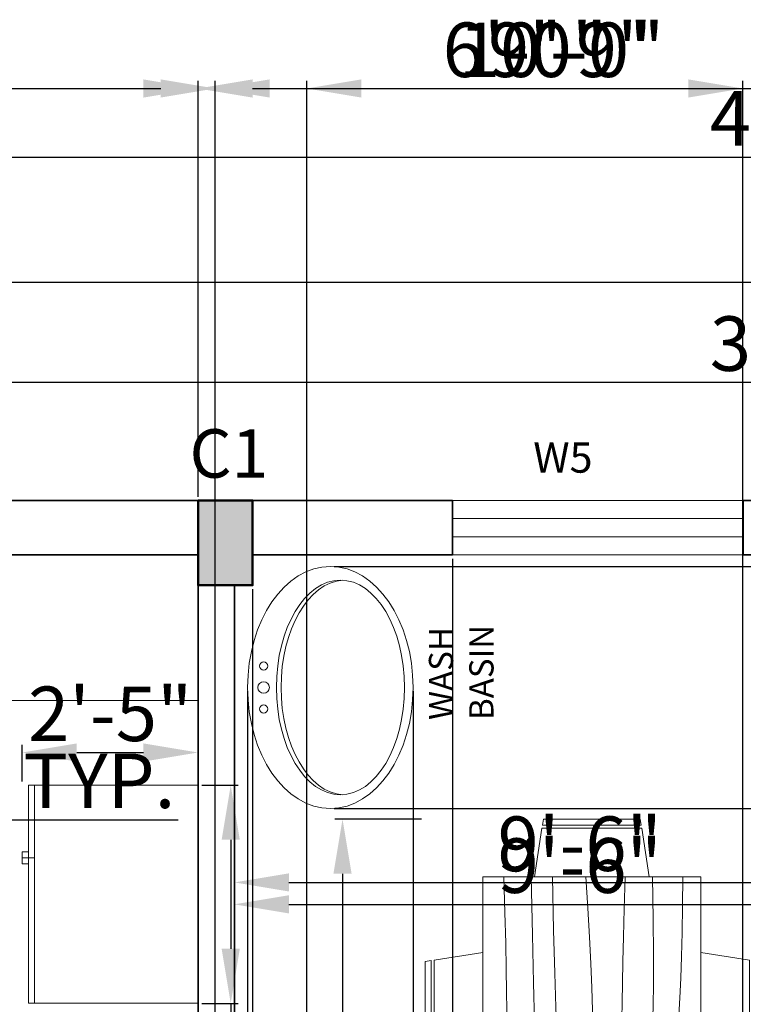
# Model space of a CAD drawing. Units: inches. Extents: x 2621 to 6190, y 513 to 1320.
# Tile 5 of 11: x 2878 to 2997, y 1003 to 1165. Entities that reach past the tile are written whole.
import ezdxf

# ---------------------------------------------------------------- set-up
doc = ezdxf.new("R2010")
doc.units = ezdxf.units.IN
for name, color, linetype, lineweight in [('A-ANNO-DIMS', 5, 'Continuous', 18), ('A-ANNO-TEXT', 7, 'Continuous', 18), ('A-EQPM', 30, 'Continuous', 13), ('A-FLOR-CASE', 30, 'Continuous', 18), ('A-FLOR-FIXT', 30, 'Continuous', 18), ('A-WALL', 7, 'Continuous', 35), ('C-PROP', 7, 'Continuous', 25), ('columns', 2, 'Continuous', 50), ('furniture', 30, 'Continuous', 18), ('S-COLS-IDEN', 2, 'Continuous', 25), ('S-COLS-PATT', 2, 'Continuous', 13), ('window', 172, 'Continuous', 18)]:
    doc.layers.add(name, color=color, linetype=linetype, lineweight=lineweight)
doc.styles.get("Standard").update_dxf_attribs({"font": 'arial.ttf'})
doc.dimstyles.new('ISO-25', dxfattribs={"dimtxt": 9, "dimasz": 9, "dimexe": 1.25, "dimexo": 0.625, "dimtad": 1, "dimlunit": 3, "dimtxsty": 'Standard', "dimcen": 2.5, "dimadec": 0, "dimazin": 0, "dimtfac": 1, "dimtmove": 0, "dimatfit": 3, "dimfxl": 1, "dimarcsym": 0})

# ---------------------------------------------------------------- blocks, each defined once
blk = doc.blocks.new('Dining Set - 36 x 72 in.')
for p, q in [((-22, 27.5), (-22.1562, 26.50042)), ((-5.8416, 26.5), (-22.1534, 26.5)), ((-22, 27.5), (-6, 27.5)), ((-5.8437, 26.49966), (-6, 27.5)), ((6, 27.5), (5.8438, 26.50042)), ((22.1584, 26.5), (5.8466, 26.5)), ((6, 27.5), (22, 27.5)), ((22.1563, 26.49966), (22, 27.5)), ((-22.2343, 26.00059), (-23.4847, 17.99762)), ((-22.2304, 26), (-5.7608, 26)), ((-4.5152, 17.99762), (-5.7655, 25.99926)), ((5.7657, 26.00059), (4.5153, 17.99762)), ((5.7696, 26), (22.2392, 26)), ((23.4848, 17.99762), (22.2345, 25.99926)), ((36, 18), (-36, 18)), ((-36, 18), (-36, -18)), ((36, -18), (36, 18)), ((-45.5, 8), (-44.5004, 8.15617)), ((-44.5, -8.15843), (-44.5, 8.15338)), ((-44.0006, 8.23428), (-35.9976, 9.48474)), ((-44, 8.23041), (-44, -8.23915)), ((44.0006, 8.23428), (35.9976, 9.48474)), ((44, 8.23041), (44, -8.23915)), ((44.5, -8.15843), (44.5, 8.15338)), ((45.5, 8), (44.5005, 8.15617)), ((-45.5, 8), (-45.5, -8)), ((45.5, 8), (45.5, -8)), ((-44.4997, -8.15631), (-45.5, -8)), ((44.4997, -8.15631), (45.5, -8)), ((-35.9976, -9.48476), (-43.9993, -8.2345)), ((35.9976, -9.48476), (43.9993, -8.2345)), ((-36, -18), (36, -18)), ((-22.2343, -26.0006), (-23.4847, -17.99762)), ((-4.5152, -17.99762), (-5.7655, -25.99928)), ((5.7657, -26.0006), (4.5153, -17.99762)), ((23.4848, -17.99762), (22.2345, -25.99928)), ((-22.2304, -26), (-5.7608, -26)), ((5.7696, -26), (22.2392, -26)), ((-22, -27.5), (-22.1562, -26.50044)), ((-5.8416, -26.5), (-22.1534, -26.5)), ((-22, -27.5), (-6, -27.5)), ((-5.8437, -26.49967), (-6, -27.5)), ((6, -27.5), (5.8438, -26.50044)), ((22.1584, -26.5), (5.8466, -26.5)), ((6, -27.5), (22, -27.5)), ((22.1563, -26.49967), (22, -27.5))]:
    blk.add_line(p, q)
for points in [[(-36, 15), (-31.1772, 14.97754), (-26.8079, 14.91406), (-22.8538, 14.81543), (-19.276, 14.6875), (-16.0362, 14.53613), (-13.0957, 14.36718), (-10.4159, 14.18652), (-7.9583, 14), (-5.6904, 13.81315), (-3.6035, 13.63021), (-1.6954, 13.45508), (0.0365, 13.29166), (1.5945, 13.14388), (2.9811, 13.01562), (4.1988, 12.9108), (5.25, 12.83333), (6.1393, 12.78613), (6.8802, 12.76823), (7.4883, 12.77767), (7.9792, 12.8125), (8.3685, 12.87077), (8.6719, 12.95052), (8.9049, 13.0498), (9.0833, 13.16666), (9.2205, 13.29899), (9.3216, 13.44401), (9.3895, 13.59879), (9.4271, 13.76041), (9.4373, 13.92594), (9.4232, 14.09245), (9.3875, 14.257), (9.3333, 14.41666), (9.2638, 14.56917), (9.1836, 14.71484), (9.0975, 14.85465), (9.0104, 14.98958), (8.9272, 15.1206), (8.8529, 15.2487), (8.7922, 15.37483), (8.75, 15.5), (8.7305, 15.62467), (8.7344, 15.74739), (8.7617, 15.86621), (8.8125, 15.97916), (8.8867, 16.08431), (8.9844, 16.17968), (9.1055, 16.26334), (9.25, 16.33333), (9.4189, 16.38802), (9.6172, 16.42708), (9.8506, 16.45052), (10.125, 16.45833), (10.4463, 16.45052), (10.8203, 16.42708), (11.2529, 16.38802), (11.75, 16.33333), (12.3184, 16.26318), (12.9694, 16.17838), (13.7151, 16.07991), (14.5677, 15.96875), (15.5395, 15.84586), (16.6426, 15.71224), (17.8893, 15.56884), (19.2917, 15.41666), (20.859, 15.25667), (22.5879, 15.08984), (24.4721, 14.91715), (26.5052, 14.73958), (28.6809, 14.5581), (30.9929, 14.3737), (33.4347, 14.18733), (36, 14)], [(-36, 10), (-28.9766, 10.14274), (-23.1725, 10.20442), (-18.4241, 10.19775), (-14.5677, 10.13541), (-11.4399, 10.03011), (-8.877, 9.89453), (-6.7154, 9.74137), (-4.7917, 9.58333), (-2.9698, 9.43082), (-1.2246, 9.28515), (0.4415, 9.14534), (2.026, 9.01041), (3.5266, 8.87939), (4.9408, 8.7513), (6.266, 8.62516), (7.5, 8.5), (8.6411, 8.37549), (9.6914, 8.2539), (10.6538, 8.13818), (11.5312, 8.03125), (12.3267, 7.93603), (13.043, 7.85547), (13.6831, 7.79248), (14.25, 7.75), (14.7471, 7.7303), (15.1797, 7.73307), (15.5537, 7.75732), (15.875, 7.80208), (16.1494, 7.86637), (16.3828, 7.94922), (16.5811, 8.04964), (16.75, 8.16666), (16.8944, 8.29915), (17.0143, 8.44531), (17.1089, 8.60319), (17.1771, 8.77083), (17.218, 8.94629), (17.2305, 9.1276), (17.2137, 9.31282), (17.1667, 9.5), (17.0895, 9.6875), (16.987, 9.875), (16.8649, 10.0625), (16.7292, 10.25), (16.5856, 10.4375), (16.4401, 10.625), (16.2985, 10.8125), (16.1667, 11), (16.05, 11.18733), (15.9518, 11.3737), (15.8752, 11.5581), (15.8229, 11.73958), (15.798, 11.91715), (15.8034, 12.08984), (15.842, 12.25667), (15.9167, 12.41666), (16.0295, 12.56836), (16.1784, 12.70833), (16.3605, 12.83268), (16.5729, 12.9375), (16.8127, 13.01888), (17.0768, 13.07291), (17.3625, 13.0957), (17.6667, 13.08333), (17.9894, 13.03312), (18.3418, 12.94726), (18.7382, 12.82918), (19.1927, 12.68229), (19.7195, 12.51001), (20.3327, 12.31575), (21.0465, 12.10294), (21.875, 11.875), (22.8357, 11.63354), (23.959, 11.37304), (25.2786, 11.08618), (26.8282, 10.76562), (28.6414, 10.40405), (30.752, 9.99414), (33.1936, 9.52856), (36, 9)], [(-36, 5.5), (-30.7157, 5.3348), (-26.069, 5.20963), (-21.9946, 5.11767), (-18.4271, 5.05208), (-15.3009, 5.00602), (-12.5508, 4.97265), (-10.1112, 4.94515), (-7.9167, 4.91666), (-5.909, 4.88167), (-4.0586, 4.83984), (-2.3429, 4.79215), (-0.7396, 4.73958), (0.7739, 4.6831), (2.22, 4.6237), (3.6213, 4.56233), (5, 4.5), (6.373, 4.43782), (7.7344, 4.3776), (9.0723, 4.32129), (10.375, 4.27083), (11.6309, 4.22819), (12.8281, 4.19531), (13.9551, 4.17415), (15, 4.16666), (15.954, 4.17448), (16.819, 4.19791), (17.6001, 4.23698), (18.3021, 4.29166), (18.9299, 4.36198), (19.4883, 4.44791), (19.9823, 4.54948), (20.4167, 4.66666), (20.7969, 4.79899), (21.1302, 4.94401), (21.4245, 5.09879), (21.6875, 5.26041), (21.9271, 5.42594), (22.1511, 5.59245), (22.3672, 5.757), (22.5834, 5.91666), (22.8065, 6.06868), (23.0404, 6.21093), (23.2879, 6.34147), (23.5521, 6.45833), (23.8358, 6.55957), (24.142, 6.64323), (24.4735, 6.70735), (24.8334, 6.75), (25.2235, 6.76969), (25.642, 6.76692), (26.0858, 6.74267), (26.5521, 6.69791), (27.0379, 6.63362), (27.5404, 6.55078), (28.0565, 6.45036), (28.5834, 6.33333), (29.1242, 6.19987), (29.7071, 6.04687), (30.3661, 5.87044), (31.1354, 5.66666), (32.0493, 5.43164), (33.142, 5.16146), (34.4475, 4.85221), (36, 4.5)], [(-36, -1), (-30.7915, -0.6591), (-26.0195, -0.38216), (-21.6519, -0.16284), (-17.6563, 0.00521), (-14.0005, 0.12833), (-10.6523, 0.21289), (-7.5796, 0.26522), (-4.75, 0.29166), (-2.134, 0.29793), (0.2878, 0.28711), (2.5317, 0.26163), (4.6146, 0.22396), (6.5529, 0.17651), (8.3633, 0.12174), (10.0623, 0.06209), (11.6667, 0), (13.1899, -0.06201), (14.6341, -0.1211), (15.9982, -0.17432), (17.2813, -0.21875), (18.4823, -0.25147), (19.6003, -0.26953), (20.6343, -0.27002), (21.5834, -0.25), (22.4481, -0.20768), (23.2357, -0.14584), (23.9549, -0.06836), (24.6146, 0.02083), (25.2235, 0.11784), (25.7904, 0.21875), (26.3241, 0.31966), (26.8334, 0.41666), (27.3265, 0.50618), (27.8099, 0.58593), (28.2894, 0.65397), (28.7709, 0.70833), (29.2601, 0.74707), (29.763, 0.76823), (30.2855, 0.76985), (30.8334, 0.75), (31.4088, 0.70784), (31.9994, 0.64713), (32.589, 0.57275), (33.1615, 0.48958), (33.7008, 0.4025), (34.1908, 0.3164), (34.6153, 0.23616), (34.9584, 0.16666), (35.2099, 0.11165), (35.3848, 0.07031), (35.504, 0.04069), (35.5886, 0.02083), (35.6594, 0.00879), (35.7377, 0.0026), (35.8442, 0.00032), (36, 0)], [(-36, -6.5), (-27.1843, -6.31267), (-20.084, -6.1263), (-14.469, -5.9419), (-10.1094, -5.76042), (-6.7752, -5.58285), (-4.2363, -5.41016), (-2.2629, -5.24333), (-0.625, -5.08334), (0.8708, -4.93099), (2.2715, -4.78646), (3.5872, -4.64974), (4.8281, -4.52084), (6.0046, -4.39974), (7.127, -4.28646), (8.2053, -4.18099), (9.25, -4.08334), (10.2705, -3.99382), (11.2734, -3.91407), (12.2647, -3.84603), (13.25, -3.79167), (14.2354, -3.75293), (15.2266, -3.73177), (16.2295, -3.73015), (17.25, -3.75), (18.2912, -3.79248), (19.3451, -3.85547), (20.4009, -3.93604), (21.4479, -4.03125), (22.4754, -4.13819), (23.4727, -4.25391), (24.4289, -4.37549), (25.3334, -4.5), (26.1785, -4.62492), (26.9694, -4.74935), (27.7145, -4.87281), (28.4219, -4.99479), (29.1, -5.11483), (29.7572, -5.23242), (30.4016, -5.34709), (31.0417, -5.45834), (31.6837, -5.56437), (32.3262, -5.65821), (32.9658, -5.73153), (33.599, -5.77604), (34.2224, -5.78345), (34.8327, -5.74545), (35.4264, -5.65373), (36, -5.5)], [(-36, -10), (-26.4022, -9.81299), (-18.4675, -9.62891), (-11.9839, -9.45069), (-6.7396, -9.28125), (-2.5226, -9.12354), (0.8789, -8.98047), (3.6769, -8.85498), (6.0833, -8.75), (8.2767, -8.66765), (10.3021, -8.60677), (12.1712, -8.56543), (13.8958, -8.54167), (15.4876, -8.53353), (16.9583, -8.53907), (18.3197, -8.55632), (19.5834, -8.58334), (20.7616, -8.61841), (21.8685, -8.66081), (22.9188, -8.71004), (23.9271, -8.76563), (24.9081, -8.82707), (25.8763, -8.89388), (26.8465, -8.96558), (27.8334, -9.04167), (28.8474, -9.12118), (29.8828, -9.20117), (30.93, -9.27824), (31.9792, -9.34896), (33.0205, -9.40991), (34.0443, -9.45768), (35.0407, -9.48885), (36, -9.5)], [(-36, -14.5), (-30.0881, -14.33513), (-25.0332, -14.21224), (-20.7312, -14.12647), (-17.0781, -14.07292), (-13.97, -14.04671), (-11.3027, -14.04297), (-8.9724, -14.05681), (-6.875, -14.08334), (-4.9224, -14.11833), (-3.0905, -14.16016), (-1.3709, -14.20785), (0.2448, -14.26042), (1.7647, -14.3169), (3.1973, -14.3763), (4.5507, -14.43767), (5.8333, -14.5), (7.0554, -14.5621), (8.235, -14.62175), (9.3922, -14.67652), (10.5469, -14.72396), (11.7192, -14.76164), (12.929, -14.78711), (14.1965, -14.79794), (15.5417, -14.79167), (16.9933, -14.76424), (18.6152, -14.70508), (20.4804, -14.60197), (22.6615, -14.44271), (25.2312, -14.21509), (28.2624, -13.9069), (31.8277, -13.50594), (36, -13)]]:
    blk.add_lwpolyline(points)
blk = doc.blocks.new('Refrigerator-2 door - 36 in top')
for p, q in [((0, -26.999999), (36, -26.999999)), ((12, -26.999999), (12, -28.999999)), ((11, -27.999999), (11, -28.999999)), ((11, -28.999999), (13, -28.999999)), ((13, -28.999999), (13, -27.999999))]:
    blk.add_line(p, q)
blk.add_lwpolyline([(0, -27.999999), (0, 0), (36, 0), (36, -27.999999)], close=True)
blk = doc.blocks.new('*D20')
at = {"layer": 'A-ANNO-DIMS', "color": 0, "lineweight": -2, "transparency": 16777216}
for p, q in [((2913.38, 1018.55), (2913.38, 1020.48)), ((2922.38, 1019.23), (3018.38, 1019.23)), ((3027.38, 1018.55), (3027.38, 1020.48))]:
    blk.add_line(p, q, dxfattribs=at)
at = {"layer": 'A-ANNO-DIMS', "color": 0, "transparency": 16777216}
for points in [[(2922.38, 1020.73), (2922.38, 1017.73), (2913.38, 1019.23)], [(3018.38, 1020.73), (3018.38, 1017.73), (3027.38, 1019.23)]]:
    blk.add_solid(points, dxfattribs=at)
at = {"layer": 'Defpoints', "color": 0, "transparency": 16777216}
for p in [(3027.38, 1019.23), (2913.38, 1017.92), (3027.38, 1017.92)]:
    blk.add_point(p, dxfattribs=at)
at = {"layer": 'A-ANNO-DIMS', "color": 0, "transparency": 16777216, "insert": (2970.38, 1024.45), "char_height": 9, "attachment_point": 5}
blk.add_mtext('9\'-6"', dxfattribs=at)
blk = doc.blocks.new('*D21')
at = {"layer": 'A-ANNO-DIMS', "color": 0, "lineweight": -2, "transparency": 16777216}
for p, q in [((2913.38, 1022.82), (2913.38, 1024.1)), ((3027.38, 1022.82), (3027.38, 1024.1)), ((2922.38, 1022.85), (3018.38, 1022.85))]:
    blk.add_line(p, q, dxfattribs=at)
at = {"layer": 'A-ANNO-DIMS', "color": 0, "transparency": 16777216}
for points in [[(2922.38, 1024.35), (2922.38, 1021.35), (2913.38, 1022.85)], [(3018.38, 1024.35), (3018.38, 1021.35), (3027.38, 1022.85)]]:
    blk.add_solid(points, dxfattribs=at)
at = {"layer": 'Defpoints', "color": 0, "transparency": 16777216}
for p in [(3027.38, 1022.85), (2913.38, 1022.19), (3027.38, 1022.19)]:
    blk.add_point(p, dxfattribs=at)
at = {"layer": 'A-ANNO-DIMS', "color": 0, "transparency": 16777216, "insert": (2970.38, 1028.07), "char_height": 9, "attachment_point": 5}
blk.add_mtext('9\'-6"', dxfattribs=at)
blk = doc.blocks.new('*D36')
at = {"layer": 'A-ANNO-DIMS', "color": 0, "lineweight": -2, "transparency": 16777216}
for p, q in [((2778.38, 1086.51), (2778.38, 1106.64)), ((2787.38, 1105.39), (3213.38, 1105.39)), ((3222.38, 1086.51), (3222.38, 1106.64))]:
    blk.add_line(p, q, dxfattribs=at)
at = {"layer": 'A-ANNO-DIMS', "color": 0, "transparency": 16777216}
for points in [[(2787.38, 1106.89), (2787.38, 1103.89), (2778.38, 1105.39)], [(3213.38, 1106.89), (3213.38, 1103.89), (3222.38, 1105.39)]]:
    blk.add_solid(points, dxfattribs=at)
at = {"layer": 'Defpoints', "color": 0, "transparency": 16777216}
for p in [(3222.38, 1105.39), (2778.38, 1085.89), (3222.38, 1085.89)]:
    blk.add_point(p, dxfattribs=at)
at = {"layer": 'A-ANNO-DIMS', "color": 0, "transparency": 16777216, "insert": (3000.38, 1110.61), "char_height": 9, "attachment_point": 5}
blk.add_mtext("37'", dxfattribs=at)
blk = doc.blocks.new('*D38')
at = {"layer": 'A-ANNO-DIMS', "color": 0, "lineweight": -2, "transparency": 16777216}
for p, q in [((2742.38, 1122.51), (2742.38, 1143.81)), ((2751.38, 1142.56), (3249.38, 1142.56)), ((3258.38, 1122.51), (3258.38, 1143.81))]:
    blk.add_line(p, q, dxfattribs=at)
at = {"layer": 'A-ANNO-DIMS', "color": 0, "transparency": 16777216}
for points in [[(2751.38, 1144.06), (2751.38, 1141.06), (2742.38, 1142.56)], [(3249.38, 1144.06), (3249.38, 1141.06), (3258.38, 1142.56)]]:
    blk.add_solid(points, dxfattribs=at)
at = {"layer": 'Defpoints', "color": 0, "transparency": 16777216}
for p in [(3258.38, 1142.56), (2742.38, 1121.89), (3258.38, 1121.89)]:
    blk.add_point(p, dxfattribs=at)
at = {"layer": 'A-ANNO-DIMS', "color": 0, "transparency": 16777216, "insert": (3000.38, 1147.79), "char_height": 9, "attachment_point": 5}
blk.add_mtext("43'", dxfattribs=at)
blk = doc.blocks.new('WIN-48IN')
for p, q in [((48, 9), (0, 9)), ((0, 9), (0, 0)), ((48, 0), (48, 9)), ((0, 6), (48, 6)), ((0, 3), (48, 3)), ((0, 0), (48, 0))]:
    blk.add_line(p, q)
blk = doc.blocks.new('COL-C1-9X14')
blk.add_lwpolyline([(0, 0), (0, 9), (14, 9), (14, 0)], close=True)
blk = doc.blocks.new('*D68')
at = {"layer": 'A-ANNO-DIMS', "color": 0, "lineweight": -2, "transparency": 16777216}
for p, q in [((2807.53, 1033.24), (2807.53, 1034.43)), ((2809.04, 1033.24), (2809.04, 1034.43)), ((2798.53, 1033.18), (2789.53, 1033.18)), ((2807.53, 1033.18), (2809.04, 1033.18)), ((2818.04, 1033.18), (2904.12, 1033.18))]:
    blk.add_line(p, q, dxfattribs=at)
at = {"layer": 'A-ANNO-DIMS', "color": 0, "transparency": 16777216}
for points in [[(2798.53, 1034.68), (2798.53, 1031.68), (2807.53, 1033.18)], [(2818.04, 1034.68), (2818.04, 1031.68), (2809.04, 1033.18)]]:
    blk.add_solid(points, dxfattribs=at)
at = {"layer": 'Defpoints', "color": 0, "transparency": 16777216}
for p in [(2807.53, 1032.61), (2809.04, 1033.18), (2809.04, 1032.61)]:
    blk.add_point(p, dxfattribs=at)
at = {"layer": 'A-ANNO-DIMS', "color": 0, "transparency": 16777216, "insert": (2865.58, 1038.46), "char_height": 9, "attachment_point": 5}
blk.add_mtext('0\'-1 1/2" TYP.', dxfattribs=at)
blk = doc.blocks.new('*D73')
at = {"layer": 'A-ANNO-DIMS', "color": 0, "lineweight": -2, "transparency": 16777216}
for p, q in [((2944.26, 1033.29), (2929.98, 1033.29)), ((2931.23, 1024.29), (2931.23, 951.29)), ((2944.26, 942.29), (2929.98, 942.29)), ((2931.23, 942.29), (2931.23, 833.12))]:
    blk.add_line(p, q, dxfattribs=at)
at = {"layer": 'A-ANNO-DIMS', "color": 0, "transparency": 16777216}
for points in [[(2929.73, 1024.29), (2932.73, 1024.29), (2931.23, 1033.29)], [(2929.73, 951.29), (2932.73, 951.29), (2931.23, 942.29)]]:
    blk.add_solid(points, dxfattribs=at)
at = {"layer": 'Defpoints', "color": 0, "transparency": 16777216}
for p in [(2944.88, 1033.29), (2931.23, 942.29), (2944.88, 942.29)]:
    blk.add_point(p, dxfattribs=at)
at = {"layer": 'A-ANNO-DIMS', "color": 0, "transparency": 16777216, "insert": (2925.95, 883.21), "char_height": 9, "attachment_point": 5, "rotation": 90}
blk.add_mtext('DINING SET 7\'-7"', dxfattribs=at)
blk = doc.blocks.new('*D75')
at = {"layer": 'A-ANNO-DIMS', "color": 0, "lineweight": -2, "transparency": 16777216}
for p, q in [((2908.01, 1038.89), (2914.03, 1038.89)), ((2912.78, 1029.89), (2912.78, 1011.89)), ((2908.01, 1002.89), (2914.03, 1002.89)), ((2912.78, 1002.89), (2912.78, 918.24))]:
    blk.add_line(p, q, dxfattribs=at)
at = {"layer": 'A-ANNO-DIMS', "color": 0, "transparency": 16777216}
for points in [[(2911.28, 1029.89), (2914.28, 1029.89), (2912.78, 1038.89)], [(2911.28, 1011.89), (2914.28, 1011.89), (2912.78, 1002.89)]]:
    blk.add_solid(points, dxfattribs=at)
at = {"layer": 'Defpoints', "color": 0, "transparency": 16777216}
for p in [(2907.38, 1038.89), (2907.38, 1002.89), (2912.78, 1002.89)]:
    blk.add_point(p, dxfattribs=at)
at = {"layer": 'A-ANNO-DIMS', "color": 0, "transparency": 16777216, "insert": (2907.5, 956.07), "char_height": 9, "attachment_point": 5, "rotation": 90}
blk.add_mtext('FRIDGE 3\'-0"', dxfattribs=at)
blk = doc.blocks.new('*D76')
at = {"layer": 'A-ANNO-DIMS', "color": 0, "lineweight": -2, "transparency": 16777216}
for p, q in [((2878.38, 1039.52), (2878.38, 1045.54)), ((2907.38, 1039.52), (2907.38, 1045.54)), ((2887.38, 1044.29), (2898.38, 1044.29))]:
    blk.add_line(p, q, dxfattribs=at)
at = {"layer": 'A-ANNO-DIMS', "color": 0, "transparency": 16777216}
for points in [[(2887.38, 1045.79), (2887.38, 1042.79), (2878.38, 1044.29)], [(2898.38, 1045.79), (2898.38, 1042.79), (2907.38, 1044.29)]]:
    blk.add_solid(points, dxfattribs=at)
at = {"layer": 'Defpoints', "color": 0, "transparency": 16777216}
for p in [(2907.38, 1044.29), (2878.38, 1038.89), (2907.38, 1038.89)]:
    blk.add_point(p, dxfattribs=at)
at = {"layer": 'A-ANNO-DIMS', "color": 0, "transparency": 16777216, "insert": (2892.88, 1049.51), "char_height": 9, "attachment_point": 5}
blk.add_mtext('2\'-5"', dxfattribs=at)
blk = doc.blocks.new('*D79')
at = {"layer": 'A-ANNO-DIMS', "color": 0, "lineweight": -2, "transparency": 16777216}
for p, q in [((2778.38, 1086.51), (2778.38, 1155.14)), ((2787.38, 1153.89), (2898.38, 1153.89)), ((2907.38, 1086.51), (2907.38, 1155.14))]:
    blk.add_line(p, q, dxfattribs=at)
at = {"layer": 'A-ANNO-DIMS', "color": 0, "transparency": 16777216}
for points in [[(2787.38, 1155.39), (2787.38, 1152.39), (2778.38, 1153.89)], [(2898.38, 1155.39), (2898.38, 1152.39), (2907.38, 1153.89)]]:
    blk.add_solid(points, dxfattribs=at)
at = {"layer": 'Defpoints', "color": 0, "transparency": 16777216}
for p in [(2907.38, 1153.89), (2778.38, 1085.89), (2907.38, 1085.89)]:
    blk.add_point(p, dxfattribs=at)
at = {"layer": 'A-ANNO-DIMS', "color": 0, "transparency": 16777216, "insert": (2842.88, 1159.11), "char_height": 9, "attachment_point": 5}
blk.add_mtext('10\'-9"', dxfattribs=at)
blk = doc.blocks.new('*D80')
at = {"layer": 'A-ANNO-DIMS', "color": 0, "lineweight": -2, "transparency": 16777216}
for p, q in [((2907.38, 1086.51), (2907.38, 1155.14)), ((2916.38, 1153.89), (3018.38, 1153.89)), ((3027.38, 1086.51), (3027.38, 1155.14))]:
    blk.add_line(p, q, dxfattribs=at)
at = {"layer": 'A-ANNO-DIMS', "color": 0, "transparency": 16777216}
for points in [[(2916.38, 1155.39), (2916.38, 1152.39), (2907.38, 1153.89)], [(3018.38, 1155.39), (3018.38, 1152.39), (3027.38, 1153.89)]]:
    blk.add_solid(points, dxfattribs=at)
at = {"layer": 'Defpoints', "color": 0, "transparency": 16777216}
for p in [(3027.38, 1153.89), (2907.38, 1085.89), (3027.38, 1085.89)]:
    blk.add_point(p, dxfattribs=at)
at = {"layer": 'A-ANNO-DIMS', "color": 0, "transparency": 16777216, "insert": (2967.38, 1159.11), "char_height": 9, "attachment_point": 5}
blk.add_mtext('10\'-0"', dxfattribs=at)
blk = doc.blocks.new('*D87')
at = {"layer": 'A-ANNO-DIMS', "color": 0, "lineweight": -2, "transparency": 16777216}
for p, q in [((2778.38, 897.51), (2778.38, 1155.14)), ((2787.38, 1153.89), (2901.22, 1153.89)), ((2910.22, 898.87), (2910.22, 1155.14))]:
    blk.add_line(p, q, dxfattribs=at)
at = {"layer": 'A-ANNO-DIMS', "color": 0, "transparency": 16777216}
for points in [[(2787.38, 1155.39), (2787.38, 1152.39), (2778.38, 1153.89)], [(2901.22, 1155.39), (2901.22, 1152.39), (2910.22, 1153.89)]]:
    blk.add_solid(points, dxfattribs=at)
at = {"layer": 'Defpoints', "color": 0, "transparency": 16777216}
for p in [(2910.22, 1153.89), (2910.22, 898.24), (2778.38, 896.89)]:
    blk.add_point(p, dxfattribs=at)
at = {"layer": 'A-ANNO-DIMS', "color": 0, "transparency": 16777216, "insert": (2844.3, 1159.11), "char_height": 9, "attachment_point": 5}
blk.add_mtext('11\'-0"', dxfattribs=at)
blk = doc.blocks.new('*D88')
at = {"layer": 'A-ANNO-DIMS', "color": 0, "lineweight": -2, "transparency": 16777216}
for p, q in [((2910.22, 898.87), (2910.22, 1155.14)), ((2919.22, 1153.89), (3018.38, 1153.89)), ((3027.38, 898.01), (3027.38, 1155.14))]:
    blk.add_line(p, q, dxfattribs=at)
at = {"layer": 'A-ANNO-DIMS', "color": 0, "transparency": 16777216}
for points in [[(2919.22, 1155.39), (2919.22, 1152.39), (2910.22, 1153.89)], [(3018.38, 1155.39), (3018.38, 1152.39), (3027.38, 1153.89)]]:
    blk.add_solid(points, dxfattribs=at)
at = {"layer": 'Defpoints', "color": 0, "transparency": 16777216}
for p in [(3027.38, 1153.89), (2910.22, 898.24), (3027.38, 897.39)]:
    blk.add_point(p, dxfattribs=at)
at = {"layer": 'A-ANNO-DIMS', "color": 0, "transparency": 16777216, "insert": (2968.8, 1159.11), "char_height": 9, "attachment_point": 5}
blk.add_mtext('9\'-9"', dxfattribs=at)
blk = doc.blocks.new('*D94')
at = {"layer": 'A-ANNO-DIMS', "color": 0, "lineweight": -2, "transparency": 16777216}
for p, q in [((2925.32, 711.51), (2925.32, 1155.14)), ((2934.32, 1153.89), (2988.32, 1153.89)), ((2997.32, 711.51), (2997.32, 1155.14))]:
    blk.add_line(p, q, dxfattribs=at)
at = {"layer": 'A-ANNO-DIMS', "color": 0, "transparency": 16777216}
for points in [[(2934.32, 1155.39), (2934.32, 1152.39), (2925.32, 1153.89)], [(2988.32, 1155.39), (2988.32, 1152.39), (2997.32, 1153.89)]]:
    blk.add_solid(points, dxfattribs=at)
at = {"layer": 'Defpoints', "color": 0, "transparency": 16777216}
for p in [(2997.32, 1153.89), (2925.32, 710.89), (2997.32, 710.89)]:
    blk.add_point(p, dxfattribs=at)
at = {"layer": 'A-ANNO-DIMS', "color": 0, "transparency": 16777216, "insert": (2961.32, 1159.11), "char_height": 9, "attachment_point": 5}
blk.add_mtext('6\'-0"', dxfattribs=at)
blk = doc.blocks.new('*D102')
at = {"layer": 'A-ANNO-DIMS', "color": 0, "lineweight": -2, "transparency": 16777216}
for p, q in [((2915.57, 1054.4), (2915.57, 519.64)), ((2942.88, 1054.4), (2942.88, 519.64)), ((2924.57, 520.89), (2933.88, 520.89)), ((2942.88, 520.89), (2998.18, 520.89))]:
    blk.add_line(p, q, dxfattribs=at)
at = {"layer": 'A-ANNO-DIMS', "color": 0, "transparency": 16777216}
for points in [[(2924.57, 522.39), (2924.57, 519.39), (2915.57, 520.89)], [(2933.88, 522.39), (2933.88, 519.39), (2942.88, 520.89)]]:
    blk.add_solid(points, dxfattribs=at)
at = {"layer": 'Defpoints', "color": 0, "transparency": 16777216}
for p in [(2915.57, 1055.03), (2942.88, 1055.03), (2942.88, 520.89)]:
    blk.add_point(p, dxfattribs=at)
at = {"layer": 'A-ANNO-DIMS', "color": 0, "transparency": 16777216, "insert": (2975.03, 526.17), "char_height": 9, "attachment_point": 5}
blk.add_mtext('2\'-3 1/2"', dxfattribs=at)
blk = doc.blocks.new('*D103')
at = {"layer": 'A-ANNO-DIMS', "color": 0, "lineweight": -2, "transparency": 16777216}
for p, q in [((2929.85, 1075), (3291.63, 1075)), ((3290.38, 1044.05), (3290.38, 1066)), ((2929.85, 1035.05), (3291.63, 1035.05))]:
    blk.add_line(p, q, dxfattribs=at)
at = {"layer": 'A-ANNO-DIMS', "color": 0, "transparency": 16777216}
for points in [[(3288.88, 1066), (3291.88, 1066), (3290.38, 1075)], [(3288.88, 1044.05), (3291.88, 1044.05), (3290.38, 1035.05)]]:
    blk.add_solid(points, dxfattribs=at)
at = {"layer": 'Defpoints', "color": 0, "transparency": 16777216}
for p in [(2929.23, 1075), (3290.38, 1075), (2929.23, 1035.05)]:
    blk.add_point(p, dxfattribs=at)
at = {"layer": 'A-ANNO-DIMS', "color": 0, "transparency": 16777216, "insert": (3285.16, 1055.03), "char_height": 9, "attachment_point": 5, "rotation": 90}
blk.add_mtext('3\'-4"', dxfattribs=at)
blk = doc.blocks.new('*D106')
at = {"layer": 'A-ANNO-DIMS', "color": 0, "lineweight": -2, "transparency": 16777216}
for p, q in [((2949.38, 1076.26), (2949.38, 519.64)), ((2916.38, 1071.26), (2916.38, 519.64)), ((2925.38, 520.89), (2940.38, 520.89))]:
    blk.add_line(p, q, dxfattribs=at)
at = {"layer": 'A-ANNO-DIMS', "color": 0, "transparency": 16777216}
for points in [[(2925.38, 522.39), (2925.38, 519.39), (2916.38, 520.89)], [(2940.38, 522.39), (2940.38, 519.39), (2949.38, 520.89)]]:
    blk.add_solid(points, dxfattribs=at)
at = {"layer": 'Defpoints', "color": 0, "transparency": 16777216}
for p in [(2949.38, 1076.89), (2916.38, 1071.89), (2949.38, 520.89)]:
    blk.add_point(p, dxfattribs=at)
at = {"layer": 'A-ANNO-DIMS', "color": 0, "transparency": 16777216, "insert": (2932.88, 526.11), "char_height": 9, "attachment_point": 5}
blk.add_mtext('2\'-9"', dxfattribs=at)

msp = doc.modelspace()

# ---------------------------------------------------------------- hatches: boundary and pattern name
at = {"layer": 'S-COLS-PATT'}
h = msp.add_hatch(color=256, dxfattribs=at)
h.dxf.hatch_style = 1
h.paths.add_polyline_path([(2787.381, 1085.89), (2778.381, 1085.89), (2778.381, 1071.89), (2787.381, 1071.89)])
h.paths.add_polyline_path([(3222.381, 1085.89), (3208.381, 1085.89), (3208.381, 1076.89), (3222.381, 1076.89)])
h.paths.add_polyline_path([(3041.381, 1085.89), (3027.381, 1085.89), (3027.381, 1076.89), (3041.381, 1076.89)])
h.paths.add_polyline_path([(2916.381, 1085.89), (2907.381, 1085.89), (2907.381, 1076.89), (2916.381, 1076.89)])
h.paths.add_polyline_path([(2916.381, 1076.89), (2913.381, 1076.89), (2913.381, 1071.89), (2916.381, 1071.89)])
h.paths.add_polyline_path([(2913.381, 1076.89), (2907.381, 1076.89), (2907.381, 1071.89), (2913.381, 1071.89)])
h.paths.add_polyline_path([(2787.381, 896.89), (2778.381, 896.89), (2778.381, 882.89), (2787.381, 882.89)])
h.paths.add_polyline_path([(2924.221, 898.241), (2910.221, 898.241), (2910.221, 889.241), (2924.221, 889.241)])
h.paths.add_polyline_path([(3036.381, 896.89), (3033.381, 896.89), (3027.381, 897.385), (3027.381, 883.385), (3033.381, 883.385), (3033.381, 890.89), (3036.381, 890.89)])
h.paths.add_polyline_path([(3036.381, 890.89), (3033.381, 890.89), (3033.381, 883.385), (3036.381, 883.385)], flags=17)
h.paths.add_polyline_path([(3222.381, 897.745), (3213.381, 897.745), (3213.381, 883.745), (3222.381, 883.745)])
h.paths.add_polyline_path([(3222.381, 710.89), (3208.381, 710.89), (3208.381, 701.89), (3222.381, 701.89)])
h.paths.add_polyline_path([(3039.318, 710.89), (3021.318, 710.89), (3021.318, 701.89), (3039.318, 701.89)])
h.paths.add_polyline_path([(2796.381, 710.89), (2778.381, 710.89), (2778.381, 701.89), (2796.381, 701.89)])

# ---------------------------------------------------------------- linework, layer by layer
at = {"layer": 'A-FLOR-CASE'}
msp.add_line((2907.381, 1052.89), (2811.381, 1052.89), dxfattribs=at)
at = {"layer": 'A-FLOR-FIXT'}
for centre, radius in [((2918.211, 1058.569), 0.677), ((2918.211, 1055.025), 0.958), ((2918.211, 1051.482), 0.677)]:
    msp.add_circle(centre, radius, dxfattribs=at)
for centre, major_axis, ratio in [((2929.225, 1055.025), (0, -19.976), 0.6834321), ((2930.89, 1055.025), (0, -17.718), 0.5968312)]:
    msp.add_ellipse(centre, major_axis=major_axis, ratio=ratio, dxfattribs=at)
msp.add_ellipse((2931.668, 1055.025), major_axis=(0, -17.718), ratio=0.5968312, start_param=3.1783849, end_param=6.246393, dxfattribs=at)
at = {"layer": 'A-WALL'}
for p, q in [((2949.381, 1085.89), (2865.381, 1085.89)), ((2949.381, 1085.89), (2949.381, 1076.89)), ((2997.381, 1085.89), (2997.381, 1076.89)), ((3089.381, 1085.89), (2997.381, 1085.89)), ((2907.381, 1076.89), (2865.381, 1076.89)), ((2907.381, 1076.89), (2907.381, 944.89)), ((2949.381, 1076.89), (2916.381, 1076.89)), ((3089.381, 1076.89), (2997.381, 1076.89)), ((2913.381, 1071.89), (2913.381, 944.89))]:
    msp.add_line(p, q, dxfattribs=at)
at = {"layer": 'C-PROP'}
msp.add_lwpolyline([(3258.381, 552.89), (3258.381, 1121.89), (2742.381, 1121.89), (2718.381, 552.89)], close=True, dxfattribs=at)

# ---------------------------------------------------------------- block references
at = {"layer": 'A-EQPM', "rotation": 270}
msp.add_blockref('Refrigerator-2 door - 36 in top', (2907.381, 1038.894), dxfattribs=at)
at = {"layer": 'columns', "rotation": 269.9999999999969}
msp.add_blockref('COL-C1-9X14', (2907.381, 1085.89), dxfattribs=at)
at = {"layer": 'furniture', "rotation": 270}
msp.add_blockref('Dining Set - 36 x 72 in.', (2972.381, 987.791), dxfattribs=at)
at = {"layer": 'window'}
msp.add_blockref('WIN-48IN', (2949.381, 1076.89), dxfattribs=at)

# ---------------------------------------------------------------- texts
at = {"layer": 'A-ANNO-TEXT', "insert": (2962.721, 1095.476), "char_height": 5, "attachment_point": 1}
msp.add_mtext_dynamic_manual_height_columns('W5', width=21.64382, gutter_width=12.5, heights=[0], dxfattribs=at)
at = {"layer": 'A-ANNO-TEXT', "insert": (2945.485, 1049.658), "char_height": 4, "attachment_point": 1, "rotation": 90}
msp.add_mtext_dynamic_manual_height_columns('WASH\\PBASIN', width=22.39726, gutter_width=12.5, heights=[0], dxfattribs=at)
at = {"layer": 'S-COLS-IDEN', "insert": (2905.974, 1097.648), "char_height": 8, "attachment_point": 1}
msp.add_mtext_dynamic_manual_height_columns('C1', width=53.01391, gutter_width=12.5, heights=[0], dxfattribs=at)

# ---------------------------------------------------------------- dimensions: what is measured, and where the dimension line sits
at = {"layer": 'A-ANNO-DIMS'}
for base, p1, p2, override, picture, middle in [((2907.381, 1153.89), (2778.381, 1085.89), (2907.381, 1085.89), {"dimdec": 1, "dimlfac": 1, "dimrnd": 0, "dimzin": 1, "dimdsep": 46, "dimlunit": 4, "dimfrac": 2}, '*D79', (2842.881, 1159.11)), ((2910.221, 1153.89), (2778.381, 896.89), (2910.221, 898.241), {"dimdec": 1, "dimlfac": 1, "dimrnd": 0, "dimzin": 1, "dimdsep": 46, "dimlunit": 4, "dimfrac": 2}, '*D87', (2844.301, 1159.11)), ((3027.381, 1153.89), (2907.381, 1085.89), (3027.381, 1085.89), {"dimdec": 1, "dimlfac": 1, "dimrnd": 0, "dimzin": 1, "dimdsep": 46, "dimlunit": 4, "dimfrac": 2}, '*D80', (2967.381, 1159.11)), ((3027.381, 1153.89), (2910.221, 898.241), (3027.381, 897.385), {"dimdec": 1, "dimlfac": 1, "dimrnd": 0, "dimzin": 1, "dimdsep": 46, "dimlunit": 4, "dimfrac": 2}, '*D88', (2968.801, 1159.11)), ((2997.318, 1153.89), (2925.318, 710.89), (2997.318, 710.89), {"dimdec": 1, "dimlfac": 1, "dimrnd": 0, "dimzin": 1, "dimdsep": 46, "dimlunit": 4, "dimfrac": 2}, '*D94', (2961.318, 1159.11)), ((3258.381, 1142.564), (2742.381, 1121.89), (3258.381, 1121.89), {"dimclrd": 0, "dimclre": 0, "dimclrt": 0}, '*D38', (3000.381, 1147.788)), ((3222.381, 1105.387), (2778.381, 1085.89), (3222.381, 1085.89), {"dimclrd": 0, "dimclre": 0, "dimclrt": 0}, '*D36', (3000.381, 1110.61)), ((2949.381, 520.89), (2916.381, 1071.89), (2949.381, 1076.89), {"dimdec": 1, "dimlfac": 1, "dimrnd": 0, "dimzin": 1, "dimdsep": 46, "dimlunit": 4, "dimfrac": 2}, '*D106', (2932.881, 526.11)), ((2907.381, 1044.294), (2878.381, 1038.894), (2907.381, 1038.894), {"dimdec": 1, "dimlfac": 1, "dimrnd": 0, "dimzin": 1, "dimdsep": 46, "dimlunit": 4, "dimfrac": 2}, '*D76', (2892.881, 1049.514)), ((2942.877, 520.89), (2915.573, 1055.025), (2942.877, 1055.025), {"dimdec": 1, "dimlfac": 1, "dimrnd": 0, "dimzin": 1, "dimdsep": 46, "dimlunit": 4, "dimfrac": 2}, '*D102', (2975.027, 526.171)), ((3027.381, 1022.85), (2913.381, 1022.192), (3027.381, 1022.192), {"dimclrd": 0, "dimclre": 0, "dimclrt": 0}, '*D21', (2970.381, 1028.07)), ((3027.381, 1019.235), (2913.381, 1017.92), (3027.381, 1017.92), {"dimclrd": 0, "dimclre": 0, "dimclrt": 0}, '*D20', (2970.381, 1024.455))]:
    dim = msp.add_linear_dim(base=base, p1=p1, p2=p2, dimstyle='ISO-25', override=override, dxfattribs=at)
    dim.commit()
    dim.dimension.update_dxf_attribs({"geometry": picture, "text_midpoint": middle})
dim = msp.add_linear_dim(base=(3290.381, 1075.001), p1=(2929.225, 1035.049), p2=(2929.225, 1075.001), angle=90, dimstyle='ISO-25', override={"dimdec": 1, "dimlfac": 1, "dimrnd": 0, "dimzin": 1, "dimdsep": 46, "dimlunit": 4, "dimfrac": 2}, dxfattribs=at)
dim.commit()
dim.dimension.update_dxf_attribs({"geometry": '*D103', "text_midpoint": (3285.158, 1055.025)})
dim = msp.add_linear_dim(base=(2809.041, 1033.182), p1=(2807.526, 1032.614), p2=(2809.041, 1032.614), text='<> TYP.', dimstyle='ISO-25', override={"dimdec": 1, "dimlfac": 1, "dimrnd": 0, "dimzin": 1, "dimdsep": 46, "dimlunit": 4, "dimfrac": 2}, dxfattribs=at)
dim.commit()
dim.dimension.update_dxf_attribs({"geometry": '*D68', "text_midpoint": (2865.582, 1038.461)})
for base, p1, p2, text, picture, middle in [((2912.781, 1002.894), (2907.381, 1038.894), (2907.381, 1002.894), 'FRIDGE <>', '*D75', (2907.499, 956.066)), ((2931.231, 942.291), (2944.881, 1033.291), (2944.881, 942.291), 'DINING SET <>', '*D73', (2925.952, 883.206))]:
    dim = msp.add_linear_dim(base=base, p1=p1, p2=p2, angle=270, text=text, dimstyle='ISO-25', override={"dimdec": 1, "dimlfac": 1, "dimrnd": 0, "dimzin": 1, "dimdsep": 46, "dimlunit": 4, "dimfrac": 2}, dxfattribs=at)
    dim.commit()
    dim.dimension.update_dxf_attribs({"geometry": picture, "text_midpoint": middle})

doc.saveas('drawing.dxf')
